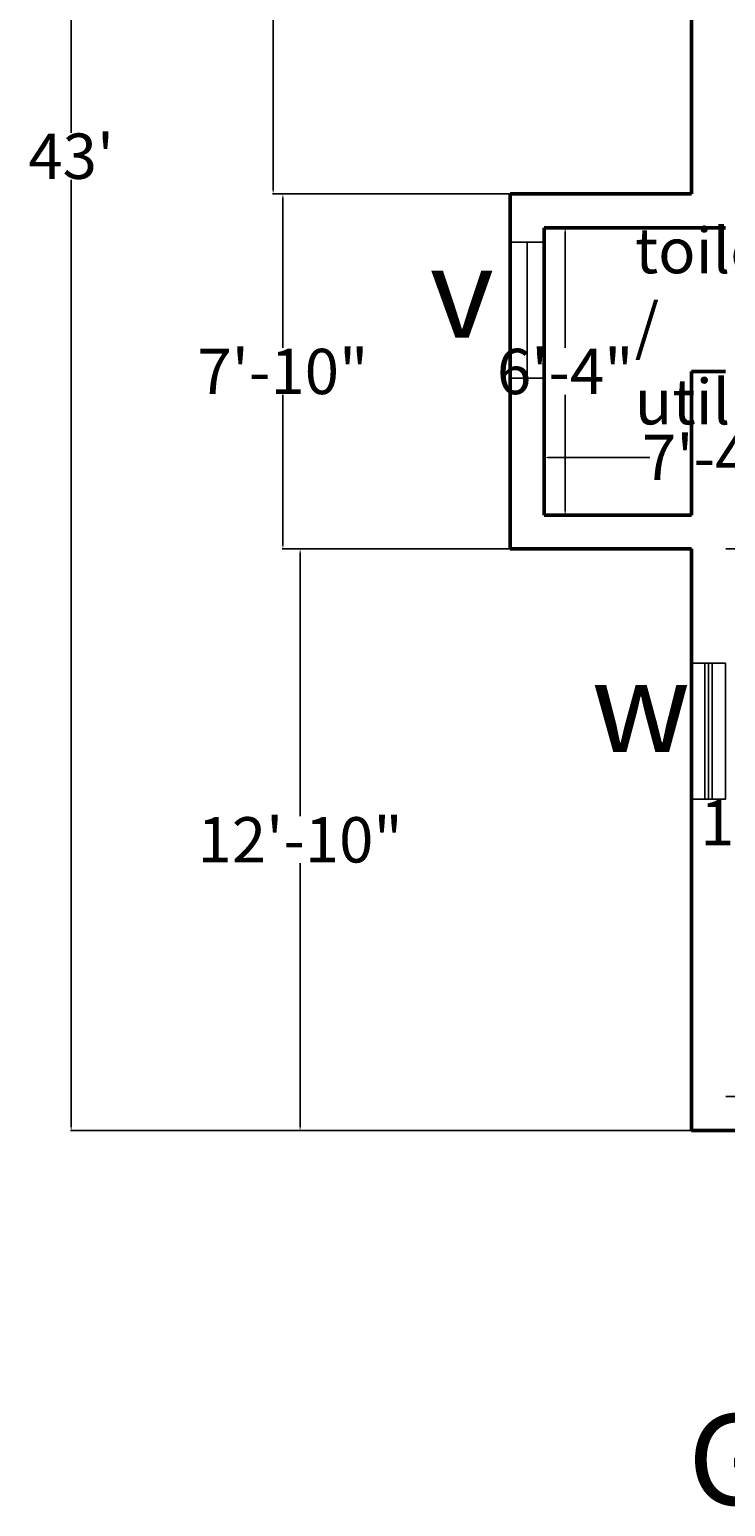
# Model space of a CAD drawing. Units: inches. Extents: x 409 to 7572, y 7 to 725.
# Tile 1 of 38: x 409 to 593, y 57 to 448. Entities that reach past the tile are written whole.
import ezdxf

# ---------------------------------------------------------------- set-up
doc = ezdxf.new("R2010")
doc.units = ezdxf.units.IN
doc.header["$MEASUREMENT"] = 0
for name, color, linetype, lineweight in [('A-ANNO-DIMS', 2, 'Continuous', 18), ('A-ANNO-SYMB', 3, 'Continuous', 25), ('A-ANNO-TEXT', 7, 'Continuous', 35), ('A-AREA-IDEN', 7, 'Continuous', 25), ('A-GLAZ', 4, 'Continuous', 25), ('A-WALL', 7, 'Continuous', 50)]:
    doc.layers.add(name, color=color, linetype=linetype, lineweight=lineweight)
doc.styles.get("Standard").update_dxf_attribs({"font": 'arial.ttf'})
doc.dimstyles.get("Standard").update_dxf_attribs({"dimtxt": 2, "dimasz": 1, "dimexe": 0.18, "dimexo": 0.0625, "dimgap": 0.09, "dimtad": 0, "dimtih": 1, "dimtoh": 1, "dimdec": 0, "dimzin": 0, "dimdsep": 46, "dimlunit": 3, "dimtxsty": 'Standard', "dimcen": 0.09, "dimadec": 0, "dimazin": 0, "dimtfac": 1, "dimtdec": 0, "dimtofl": 0, "dimtmove": 0, "dimatfit": 3, "dimfxl": 1, "dimtolj": 1, "dimtzin": 0, "dimarcsym": 0})

# ---------------------------------------------------------------- blocks, each defined once
blk = doc.blocks.new('*D18')
at = {"layer": 'A-ANNO-DIMS', "color": 0, "lineweight": -2, "transparency": 16777216}
for p, q in [((593.22, 310.53), (609.26, 310.53)), ((609.08, 309.53), (609.08, 244.15)), ((609.08, 166.53), (609.08, 231.92)), ((593.22, 165.53), (609.26, 165.53))]:
    blk.add_line(p, q, dxfattribs=at)
at = {"layer": 'A-ANNO-DIMS', "color": 0, "transparency": 16777216}
for points in [[(608.91, 309.53), (609.25, 309.53), (609.08, 310.53)], [(608.91, 166.53), (609.25, 166.53), (609.08, 165.53)]]:
    blk.add_solid(points, dxfattribs=at)
at = {"layer": 'DEFPOINTS', "color": 0, "transparency": 16777216}
for p in [(593.16, 310.53), (593.16, 165.53), (609.08, 165.53)]:
    blk.add_point(p, dxfattribs=at)
at = {"layer": 'A-ANNO-DIMS', "color": 0, "transparency": 16777216, "insert": (609.08, 238.03), "char_height": 2, "attachment_point": 5}
blk.add_mtext('\\A1;{\\H6x;12\'-1"}', dxfattribs=at)
blk = doc.blocks.new('*D27')
at = {"layer": 'A-ANNO-DIMS', "color": 0, "lineweight": -2, "transparency": 16777216}
for p, q in [((554.36, 395.53), (550.54, 395.53)), ((550.72, 394.53), (550.72, 363.75)), ((550.72, 320.53), (550.72, 351.31)), ((554.36, 319.53), (550.54, 319.53))]:
    blk.add_line(p, q, dxfattribs=at)
at = {"layer": 'A-ANNO-DIMS', "color": 0, "transparency": 16777216}
for points in [[(550.55, 394.53), (550.89, 394.53), (550.72, 395.53)], [(550.55, 320.53), (550.89, 320.53), (550.72, 319.53)]]:
    blk.add_solid(points, dxfattribs=at)
at = {"layer": 'DEFPOINTS', "color": 0, "transparency": 16777216}
for p in [(554.42, 395.53), (550.72, 319.53), (554.42, 319.53)]:
    blk.add_point(p, dxfattribs=at)
at = {"layer": 'A-ANNO-DIMS', "color": 0, "transparency": 16777216, "insert": (550.72, 357.53), "char_height": 2, "attachment_point": 5}
blk.add_mtext('\\A1;{\\H6x;6\'-4"}', dxfattribs=at)
blk = doc.blocks.new('*D29')
at = {"layer": 'A-ANNO-DIMS', "color": 0, "lineweight": -2, "transparency": 16777216}
for p, q in [((545.16, 346.33), (545.16, 334.6)), ((633.16, 346.33), (633.16, 334.6)), ((546.16, 334.78), (573.17, 334.78)), ((632.16, 334.78), (605.15, 334.78))]:
    blk.add_line(p, q, dxfattribs=at)
at = {"layer": 'A-ANNO-DIMS', "color": 0, "transparency": 16777216}
for points in [[(546.16, 334.95), (546.16, 334.61), (545.16, 334.78)], [(632.16, 334.95), (632.16, 334.61), (633.16, 334.78)]]:
    blk.add_solid(points, dxfattribs=at)
at = {"layer": 'DEFPOINTS', "color": 0, "transparency": 16777216}
for p in [(545.16, 346.39), (633.16, 346.39), (633.16, 334.78)]:
    blk.add_point(p, dxfattribs=at)
at = {"layer": 'A-ANNO-DIMS', "color": 0, "transparency": 16777216, "insert": (589.16, 334.78), "char_height": 2, "attachment_point": 5}
blk.add_mtext('\\A1;{\\H6x;7\'-4"}', dxfattribs=at)
blk = doc.blocks.new('*D31')
at = {"layer": 'A-ANNO-DIMS', "color": 0, "lineweight": -2, "transparency": 16777216}
for p, q in [((584.09, 672.53), (473.2, 672.53)), ((473.38, 671.53), (473.38, 544.65)), ((473.38, 405.53), (473.38, 532.42)), ((584.09, 404.53), (473.2, 404.53))]:
    blk.add_line(p, q, dxfattribs=at)
at = {"layer": 'A-ANNO-DIMS', "color": 0, "transparency": 16777216}
for points in [[(473.21, 671.53), (473.54, 671.53), (473.38, 672.53)], [(473.21, 405.53), (473.54, 405.53), (473.38, 404.53)]]:
    blk.add_solid(points, dxfattribs=at)
at = {"layer": 'DEFPOINTS', "color": 0, "transparency": 16777216}
for p in [(584.16, 672.53), (473.38, 404.53), (584.16, 404.53)]:
    blk.add_point(p, dxfattribs=at)
at = {"layer": 'A-ANNO-DIMS', "color": 0, "transparency": 16777216, "insert": (473.38, 538.53), "char_height": 2, "attachment_point": 5}
blk.add_mtext('\\A1;{\\H6x;22\'-4"}', dxfattribs=at)
blk = doc.blocks.new('*D32')
at = {"layer": 'A-ANNO-DIMS', "color": 0, "lineweight": -2, "transparency": 16777216}
for p, q in [((536.09, 404.53), (475.79, 404.53)), ((475.97, 403.53), (475.97, 363.75)), ((475.97, 311.53), (475.97, 351.31)), ((536.09, 310.53), (475.79, 310.53))]:
    blk.add_line(p, q, dxfattribs=at)
at = {"layer": 'A-ANNO-DIMS', "color": 0, "transparency": 16777216}
for points in [[(475.8, 403.53), (476.13, 403.53), (475.97, 404.53)], [(475.8, 311.53), (476.13, 311.53), (475.97, 310.53)]]:
    blk.add_solid(points, dxfattribs=at)
at = {"layer": 'DEFPOINTS', "color": 0, "transparency": 16777216}
for p in [(536.16, 404.53), (475.97, 310.53), (536.16, 310.53)]:
    blk.add_point(p, dxfattribs=at)
at = {"layer": 'A-ANNO-DIMS', "color": 0, "transparency": 16777216, "insert": (475.97, 357.53), "char_height": 2, "attachment_point": 5}
blk.add_mtext('\\A1;{\\H6x;7\'-10"}', dxfattribs=at)
blk = doc.blocks.new('*D33')
at = {"layer": 'A-ANNO-DIMS', "color": 0, "lineweight": -2, "transparency": 16777216}
for p, q in [((584.09, 310.53), (480.35, 310.53)), ((480.53, 309.53), (480.53, 239.75)), ((480.53, 157.53), (480.53, 227.31)), ((584.09, 156.53), (480.35, 156.53))]:
    blk.add_line(p, q, dxfattribs=at)
at = {"layer": 'A-ANNO-DIMS', "color": 0, "transparency": 16777216}
for points in [[(480.36, 309.53), (480.69, 309.53), (480.53, 310.53)], [(480.36, 157.53), (480.69, 157.53), (480.53, 156.53)]]:
    blk.add_solid(points, dxfattribs=at)
at = {"layer": 'DEFPOINTS', "color": 0, "transparency": 16777216}
for p in [(584.16, 310.53), (480.53, 156.53), (584.16, 156.53)]:
    blk.add_point(p, dxfattribs=at)
at = {"layer": 'A-ANNO-DIMS', "color": 0, "transparency": 16777216, "insert": (480.53, 233.53), "char_height": 2, "attachment_point": 5}
blk.add_mtext('\\A1;{\\H6x;12\'-10"}', dxfattribs=at)
blk = doc.blocks.new('*D34')
at = {"layer": 'A-ANNO-DIMS', "color": 0, "lineweight": -2, "transparency": 16777216}
for p, q in [((584.09, 672.53), (419.74, 672.53)), ((419.92, 671.53), (419.92, 420.75)), ((419.92, 157.53), (419.92, 408.31)), ((584.09, 156.53), (419.74, 156.53))]:
    blk.add_line(p, q, dxfattribs=at)
at = {"layer": 'A-ANNO-DIMS', "color": 0, "transparency": 16777216}
for points in [[(419.75, 671.53), (420.09, 671.53), (419.92, 672.53)], [(419.75, 157.53), (420.09, 157.53), (419.92, 156.53)]]:
    blk.add_solid(points, dxfattribs=at)
at = {"layer": 'DEFPOINTS', "color": 0, "transparency": 16777216}
for p in [(584.16, 672.53), (419.92, 156.53), (584.16, 156.53)]:
    blk.add_point(p, dxfattribs=at)
at = {"layer": 'A-ANNO-DIMS', "color": 0, "transparency": 16777216, "insert": (419.92, 414.53), "char_height": 2, "attachment_point": 5}
blk.add_mtext("\\A1;{\\H6x;43'}", dxfattribs=at)
blk = doc.blocks.new('WIN-36')
for p, q in [((1699.82, 514.65), (1699.82, 478.65)), ((1700.82, 514.65), (1700.82, 478.65)), ((1701.82, 514.65), (1701.82, 478.65))]:
    blk.add_line(p, q)
blk.add_lwpolyline([(1705.32, 514.65), (1705.32, 478.65), (1696.32, 478.65), (1696.32, 514.65)], close=True)
blk = doc.blocks.new('VENT-36')
blk.add_line((5633.28, 355.73), (5633.28, 391.73))
blk.add_lwpolyline([(5628.78, 355.73), (5628.78, 391.73), (5637.78, 391.73), (5637.78, 355.73)], close=True)

msp = doc.modelspace()

# ---------------------------------------------------------------- linework, layer by layer
at = {"layer": 'A-WALL'}
for p, q in [((584.16, 672.53), (584.16, 404.53)), ((536.16, 404.53), (536.16, 310.53)), ((584.16, 404.53), (536.16, 404.53)), ((545.16, 395.53), (545.16, 319.53)), ((593.16, 395.53), (545.16, 395.53)), ((584.16, 357.53), (584.16, 319.53)), ((593.16, 357.53), (584.16, 357.53)), ((584.16, 319.53), (545.16, 319.53)), ((584.16, 310.53), (536.16, 310.53)), ((584.16, 310.53), (584.16, 156.53)), ((584.16, 156.53), (958.16, 156.53))]:
    msp.add_line(p, q, dxfattribs=at)

# ---------------------------------------------------------------- block references
at = {"layer": 'A-GLAZ'}
for name, p in [('VENT-36', (-5092.63, 0)), ('WIN-36', (-1112.16, -234.38))]:
    msp.add_blockref(name, p, dxfattribs=at)

# ---------------------------------------------------------------- texts
at = {"layer": 'A-ANNO-SYMB', "char_height": 24, "attachment_point": 1}
for s, insert in [('v', (514.82, 390.47)), ('w', (557.63, 280.77))]:
    msp.add_mtext_dynamic_manual_height_columns(s, width=18.2582, gutter_width=1, heights=[0], dxfattribs=dict(at, insert=insert))
at = {"layer": 'A-ANNO-TEXT', "insert": (583.19, 81.45), "char_height": 24, "attachment_point": 1}
msp.add_mtext_dynamic_manual_height_columns('GROUND FLOOR', width=577.2242, gutter_width=1, heights=[0], dxfattribs=at)
at = {"layer": 'A-AREA-IDEN', "insert": (569.16, 395.53), "char_height": 12, "attachment_point": 1}
msp.add_mtext_dynamic_manual_height_columns('toilet / utility', width=49.2946, gutter_width=1, heights=[0], dxfattribs=at)

# ---------------------------------------------------------------- dimensions: what is measured, and where the dimension line sits
at = {"layer": 'A-ANNO-DIMS'}
for base, p1, p2, picture, middle in [((419.92, 156.53), (584.16, 672.53), (584.16, 156.53), '*D34', (419.92, 414.53)), ((473.38, 404.53), (584.16, 672.53), (584.16, 404.53), '*D31', (473.38, 538.53)), ((475.97, 310.53), (536.16, 404.53), (536.16, 310.53), '*D32', (475.97, 357.53)), ((550.72, 319.53), (554.42, 395.53), (554.42, 319.53), '*D27', (550.72, 357.53)), ((480.53, 156.53), (584.16, 310.53), (584.16, 156.53), '*D33', (480.53, 233.53)), ((609.08, 165.53), (593.16, 310.53), (593.16, 165.53), '*D18', (609.08, 238.03))]:
    dim = msp.add_linear_dim(base=base, p1=p1, p2=p2, angle=90, text='{\\H6x;<>}', dimstyle='Standard', override={"dimclrd": 0, "dimclre": 0, "dimclrt": 0}, dxfattribs=at)
    dim.commit()
    dim.dimension.update_dxf_attribs({"geometry": picture, "text_midpoint": middle})
dim = msp.add_linear_dim(base=(633.16, 334.78), p1=(545.16, 346.39), p2=(633.16, 346.39), text='{\\H6x;<>}', dimstyle='Standard', override={"dimclrd": 0, "dimclre": 0, "dimclrt": 0}, dxfattribs=at)
dim.commit()
dim.dimension.update_dxf_attribs({"geometry": '*D29', "text_midpoint": (589.16, 334.78)})

doc.saveas('drawing.dxf')
